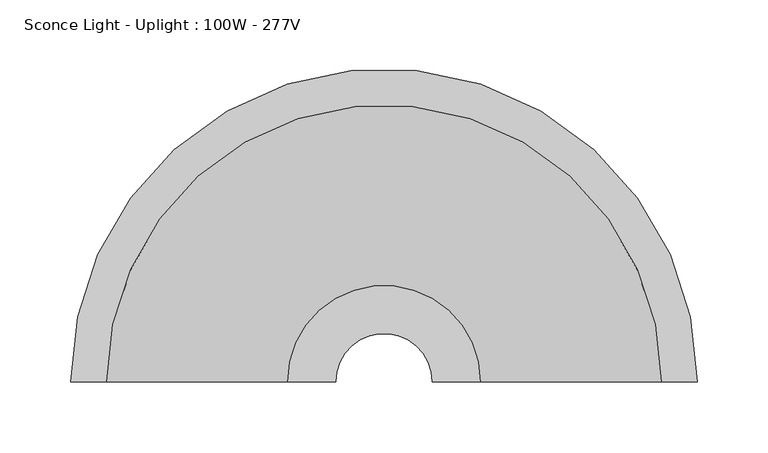
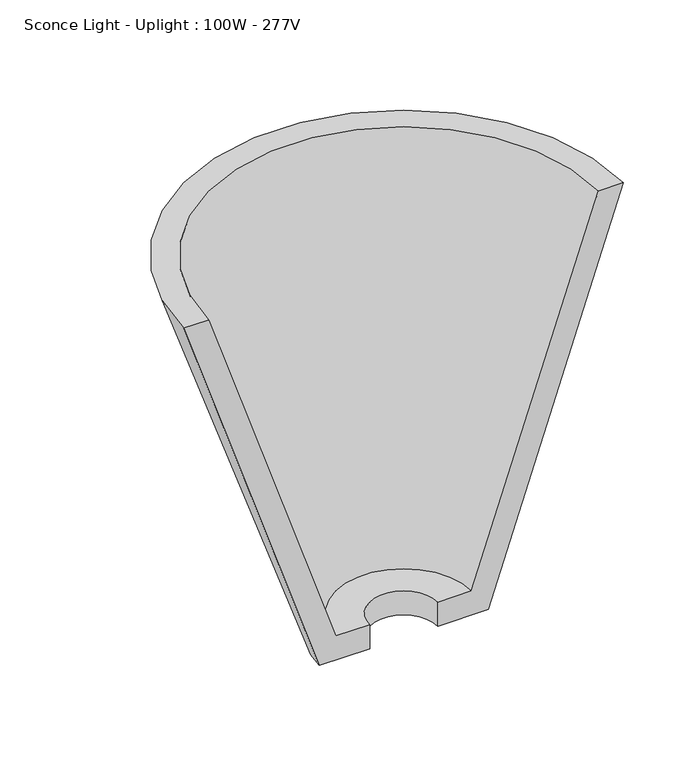
"""IFC4 building model written with IfcOpenShell, lengths in millimetres: light fixture geometry, Sconce Light - Uplight : 100W - 277V."""

from ifc_helpers import new_model, si_unit, frame, origin, place, context, project, spatial, polyline, circle_curve, source, transform, mapped, element, save
from ifc_brep_helpers import plane_surface, revolved_surface, advanced_brep


def sconce_light_uplight_100w_277v_9e84f6ed(model_context):
    return source(origin(), model_context, "Body", "AdvancedBrep", [
        advanced_brep(
        [(-221.2056669, 152.4, 2133.6), (-85.0253975, 152.4, 1727.2), (-34.2253975, 152.4, 1727.2), (-34.2253975, 152.4, 1752.6), (-68.1366644, 152.4, 1752.6), (-195.8056669, 152.4, 2133.6), (221.2056669, 152.4, 2133.6), (195.8056669, 152.4, 2133.6), (68.1366644, 152.4, 1752.6), (34.2253975, 152.4, 1752.6), (34.2253975, 152.4, 1727.2), (85.0253975, 152.4, 1727.2)],
        [
            (0, 1),
            (1, 2),
            (2, 3),
            (3, 4),
            (4, 5),
            (5, 0),
            (6, 7),
            (7, 8),
            (8, 9),
            (9, 10),
            (10, 11),
            (11, 6),
            (11, 1, circle_curve(frame((0.0, 152.4, 1727.2), z_axis=(0.0, 0.0, 1.0), x_axis=(-1.0, 0.0, 0.0)), 85.0253975)),
            (0, 6, circle_curve(frame((0.0, 152.4, 2133.6), z_axis=(0.0, 0.0, -1.0), x_axis=(-1.0, 0.0, 0.0)), 221.2056669)),
            (10, 2, circle_curve(frame((0.0, 152.4, 1727.2), z_axis=(0.0, 0.0, 1.0), x_axis=(-1.0, 0.0, 0.0)), 34.2253975)),
            (9, 3, circle_curve(frame((0.0, 152.4, 1752.6), z_axis=(0.0, 0.0, 1.0), x_axis=(-1.0, 0.0, 0.0)), 34.2253975)),
            (8, 4, circle_curve(frame((0.0, 152.4, 1752.6), z_axis=(0.0, 0.0, 1.0), x_axis=(-1.0, 0.0, 0.0)), 68.1366644)),
            (7, 5, circle_curve(frame((0.0, 152.4, 2133.6), z_axis=(0.0, 0.0, 1.0), x_axis=(-1.0, 0.0, 0.0)), 195.8056669)),
        ],
        [
            plane_surface(frame((0.0, 152.4, 1967.174367), z_axis=(0.0, -1.0, 0.0), x_axis=(-1.0, 0.0, 0.0))),
            plane_surface(frame((0.0, 152.4, 1967.174367), z_axis=(0.0, -1.0, 0.0), x_axis=(1.0, 0.0, 0.0))),
            revolved_surface(polyline([(-221.2056669, 152.4, 2133.6), (-85.0253975, 152.4, 1727.2)]), (0.0, 152.4, 1967.174367), (0.0, 0.0, -1.0)),
            plane_surface(frame((0.0, 152.4, 1727.2), z_axis=(0.0, 0.0, -1.0), x_axis=(-1.0, 0.0, 0.0))),
            revolved_surface(polyline([(-34.2253975, 152.4, 1727.2), (-34.2253975, 152.4, 1752.6)]), (0.0, 152.4, 1967.174367), (0.0, 0.0, -1.0)),
            plane_surface(frame((0.0, 152.4, 1752.6), z_axis=(0.0, 0.0, 1.0), x_axis=(-1.0, 0.0, 0.0))),
            revolved_surface(polyline([(-68.1366644, 152.4, 1752.6), (-195.8056669, 152.4, 2133.6)]), (0.0, 152.4, 1967.174367), (0.0, 0.0, -1.0)),
            plane_surface(frame((0.0, 152.4, 2133.6), z_axis=(0.0, 0.0, 1.0), x_axis=(-1.0, 0.0, 0.0))),
        ],
        [
            (0, [[1, 2, 3, 4, 5, 6]]),
            (1, [[7, 8, 9, 10, 11, 12]]),
            (2, [[13, -1, 14, -12]]),
            (3, [[15, -2, -13, -11]]),
            (4, [[16, -3, -15, -10]]),
            (5, [[17, -4, -16, -9]]),
            (6, [[18, -5, -17, -8]]),
            (7, [[-14, -6, -18, -7]]),
        ],
    ),
    ])


if __name__ == "__main__":
    model = new_model("IFC4")
    model_context = context("Model", 3, world=origin())
    ifc_project = project(units=[si_unit("LENGTHUNIT", "METRE", prefix="MILLI")], contexts=[model_context])
    site = spatial("IfcSite", under=ifc_project)
    building = spatial("IfcBuilding", under=site)
    placement = place(None, origin())
    sconce_light_uplight_100w_277v_shape = sconce_light_uplight_100w_277v_9e84f6ed(model_context)
    element("IfcLightFixture", 1, ObjectType="Sconce Light - Uplight : 100W - 277V", at=placement, inside=building, context=model_context, shape_type="MappedRepresentation", body=[
        mapped(sconce_light_uplight_100w_277v_shape, transform((0.0, 0.0, 0.0), x_axis=(1.0, 0.0, 0.0), y_axis=(0.0, 1.0, 0.0), z_axis=(0.0, 0.0, 1.0))),
    ])
    save(model, "model.ifc")

# Revit data of these elements
# Type "Sconce Light - Uplight : 100W - 277V"
#   Assembly Code = "D5020220"
#   Lamp = "R-30"
#   Wattage = 100 W
#   built-in parameter 1150110 = 1 (stored number, unit not read)
#   built-in parameter 1114217 = 1 (stored number, unit not read)
#   built-in parameter 1150109 = 1 (stored number, unit not read)
#   built-in parameter 1150113 = 1 (stored number, unit not read)
#   built-in parameter 1150115 = 1 (stored number, unit not read)
#   built-in parameter 1150105 = 381.972 (stored number, unit not read)
#   Light Source Symbol Size = 2' - 0"
#   built-in parameter 1150112 = 1 (stored number, unit not read)
#   built-in parameter 1150114 = 1 (stored number, unit not read)
#   built-in parameter 1150107 = 2800 (stored number, unit not read)
#   built-in parameter 1150106 = 3.81972 (stored number, unit not read)
#   built-in parameter 1150104 = 1.11484 (stored number, unit not read)
#   Ballast Voltage = 277 V
#   built-in parameter 1114218 = 1 (stored number, unit not read)
#   built-in parameter 1150133 = 10 (stored number, unit not read)
#   Lumens = 1200 lm
#   Mounting Height = 6' - 4"
#   Apparent Load = 100 VA
#   built-in parameter 1150134 = 4
#   built-in parameter 1150137 = 1
#   Color Filter = 16777215
#   built-in parameter 1140040 [instance default] = 1
#   Ballast Number of Poles = 1
#   Shade Material = Glass, Frosted
#   Dimming Lamp Color Temperature Shift = (empty or 0)
#   Default Elevation = 0
#   Wattage Comments = ""
# Element 1 (IfcLightFixture, "Sconce Light - Uplight : 100W - 277V")
#   Materials on its faces: "Glass, Frosted"
# Materials
#   "Glass, Frosted": class "Glass", colour RGB 250 244 225, transparency 0.55, Description = "physical material", Cost = 0
